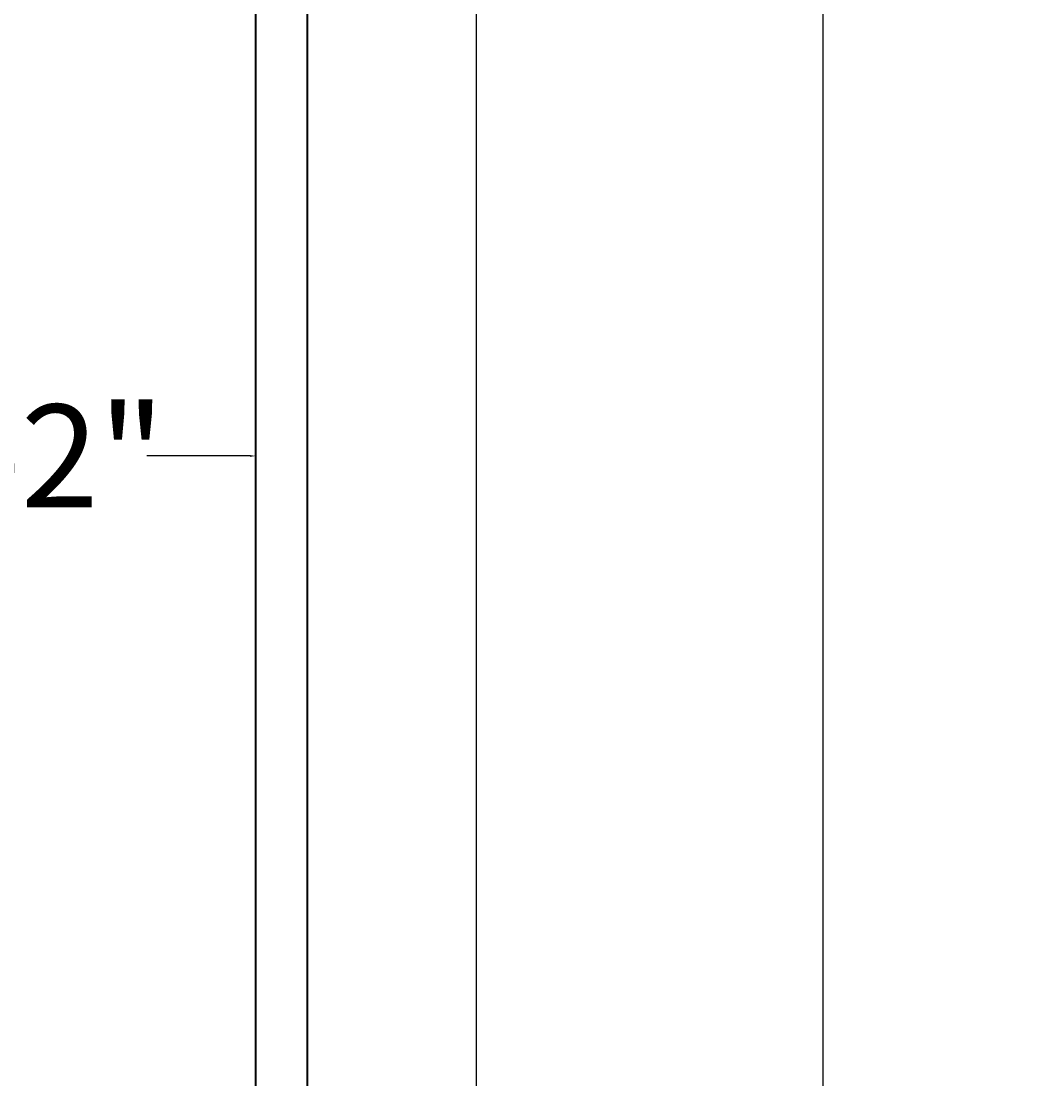
# Model space of a CAD drawing. Units: inches. Extents: x -2189 to 546, y 945 to 2684.
# Tile 8 of 10: x -313 to -134, y 2267 to 2452. Entities that reach past the tile are written whole.
import ezdxf

# ---------------------------------------------------------------- set-up
doc = ezdxf.new("R2010")
doc.units = ezdxf.units.IN
doc.header["$MEASUREMENT"] = 0
doc.layers.add('A-ANNO-DIMS', color=2, linetype='Continuous', lineweight=13)
doc.layers.add('A-WALL', color=7, linetype='Continuous', lineweight=35)
doc.styles.get("Standard").update_dxf_attribs({"font": 'arial.ttf'})
doc.dimstyles.get("Standard").update_dxf_attribs({"dimtxt": 1, "dimasz": 1, "dimexe": 0.18, "dimexo": 0.0625, "dimgap": 0.09, "dimtad": 0, "dimtih": 1, "dimtoh": 1, "dimdec": 0, "dimzin": 0, "dimdsep": 46, "dimlunit": 3, "dimtxsty": 'Standard', "dimcen": 0.09, "dimadec": 0, "dimazin": 0, "dimtfac": 1, "dimtdec": 0, "dimtofl": 0, "dimtmove": 0, "dimatfit": 3, "dimfxl": 1, "dimtolj": 1, "dimtzin": 0, "dimarcsym": 0})

# ---------------------------------------------------------------- blocks, each defined once
blk = doc.blocks.new('*D79')
at = {"layer": 'A-ANNO-DIMS', "color": 0, "lineweight": -2, "transparency": 16777216}
for p, q in [((-262.72, 2600.17), (-172.26, 2600.17)), ((-172.44, 2599.17), (-172.44, 1833.96)), ((-172.44, 1050.17), (-172.44, 1815.39)), ((-262.72, 1049.17), (-172.26, 1049.17))]:
    blk.add_line(p, q, dxfattribs=at)
at = {"layer": 'A-ANNO-DIMS', "color": 0, "transparency": 16777216}
for points in [[(-172.6, 2599.17), (-172.27, 2599.17), (-172.44, 2600.17)], [(-172.6, 1050.17), (-172.27, 1050.17), (-172.44, 1049.17)]]:
    blk.add_solid(points, dxfattribs=at)
at = {"layer": 'Defpoints', "color": 0, "transparency": 16777216}
for p in [(-262.78, 2600.17), (-172.44, 2600.17), (-262.78, 1049.17)]:
    blk.add_point(p, dxfattribs=at)
at = {"layer": 'A-ANNO-DIMS', "color": 0, "transparency": 16777216, "insert": (-172.44, 1824.67), "char_height": 1, "attachment_point": 5}
blk.add_mtext('\\A1;{\\H18x;129\'-3"}', dxfattribs=at)
blk = doc.blocks.new('*D80')
at = {"layer": 'A-ANNO-DIMS', "color": 0, "lineweight": -2, "transparency": 16777216}
for p, q in [((-271.72, 2591.17), (-233.01, 2591.17)), ((-233.19, 2590.17), (-233.19, 1833.95)), ((-233.19, 1059.17), (-233.19, 1815.39)), ((-271.72, 1058.17), (-233.01, 1058.17))]:
    blk.add_line(p, q, dxfattribs=at)
at = {"layer": 'A-ANNO-DIMS', "color": 0, "transparency": 16777216}
for points in [[(-233.36, 2590.17), (-233.03, 2590.17), (-233.19, 2591.17)], [(-233.36, 1059.17), (-233.03, 1059.17), (-233.19, 1058.17)]]:
    blk.add_solid(points, dxfattribs=at)
at = {"layer": 'Defpoints', "color": 0, "transparency": 16777216}
for p in [(-271.78, 2591.17), (-233.19, 2591.17), (-271.78, 1058.17)]:
    blk.add_point(p, dxfattribs=at)
at = {"layer": 'A-ANNO-DIMS', "color": 0, "transparency": 16777216, "insert": (-233.19, 1824.67), "char_height": 1, "attachment_point": 5}
blk.add_mtext('\\A1;{\\H18x;127\'-9"}', dxfattribs=at)
blk = doc.blocks.new('*D83')
at = {"layer": 'A-ANNO-DIMS', "color": 0, "lineweight": -2, "transparency": 16777216}
for p, q in [((-357.78, 2376.1), (-357.78, 2376.22)), ((-356.78, 2376.04), (-338.72, 2376.04)), ((-272.78, 2376.04), (-290.84, 2376.04)), ((-271.78, 2376.1), (-271.78, 2376.22))]:
    blk.add_line(p, q, dxfattribs=at)
at = {"layer": 'A-ANNO-DIMS', "color": 0, "transparency": 16777216}
for points in [[(-356.78, 2376.2), (-356.78, 2375.87), (-357.78, 2376.04)], [(-272.78, 2376.2), (-272.78, 2375.87), (-271.78, 2376.04)]]:
    blk.add_solid(points, dxfattribs=at)
at = {"layer": 'Defpoints', "color": 0, "transparency": 16777216}
for p in [(-357.78, 2376.04), (-271.78, 2376.04), (-271.78, 2376.04)]:
    blk.add_point(p, dxfattribs=at)
at = {"layer": 'A-ANNO-DIMS', "color": 0, "transparency": 16777216, "insert": (-314.78, 2376.04), "char_height": 1, "attachment_point": 5}
blk.add_mtext('\\A1;{\\H18x;7\'-2"}', dxfattribs=at)

msp = doc.modelspace()

# ---------------------------------------------------------------- linework, layer by layer
at = {"layer": 'A-WALL'}
for p, q in [((-262.78, 2600.17), (-262.78, 1049.17)), ((-271.78, 2591.17), (-271.78, 1058.17))]:
    msp.add_line(p, q, dxfattribs=at)

# ---------------------------------------------------------------- dimensions: what is measured, and where the dimension line sits
at = {"layer": 'A-ANNO-DIMS'}
for base, p1, p2, picture, middle in [((-172.44, 2600.17), (-262.78, 1049.17), (-262.78, 2600.17), '*D79', (-172.44, 1824.67)), ((-233.19, 2591.17), (-271.78, 1058.17), (-271.78, 2591.17), '*D80', (-233.19, 1824.67))]:
    dim = msp.add_linear_dim(base=base, p1=p1, p2=p2, angle=90, text='{\\H18x;<>}', dimstyle='Standard', override={"dimclrd": 0, "dimclre": 0, "dimclrt": 0}, dxfattribs=at)
    dim.commit()
    dim.dimension.update_dxf_attribs({"geometry": picture, "text_midpoint": middle})
dim = msp.add_linear_dim(base=(-271.78, 2376.04), p1=(-357.78, 2376.04), p2=(-271.78, 2376.04), text='{\\H18x;<>}', dimstyle='Standard', override={"dimclrd": 0, "dimclre": 0, "dimclrt": 0}, dxfattribs=at)
dim.commit()
dim.dimension.update_dxf_attribs({"geometry": '*D83', "text_midpoint": (-314.78, 2376.04)})

doc.saveas('drawing.dxf')
